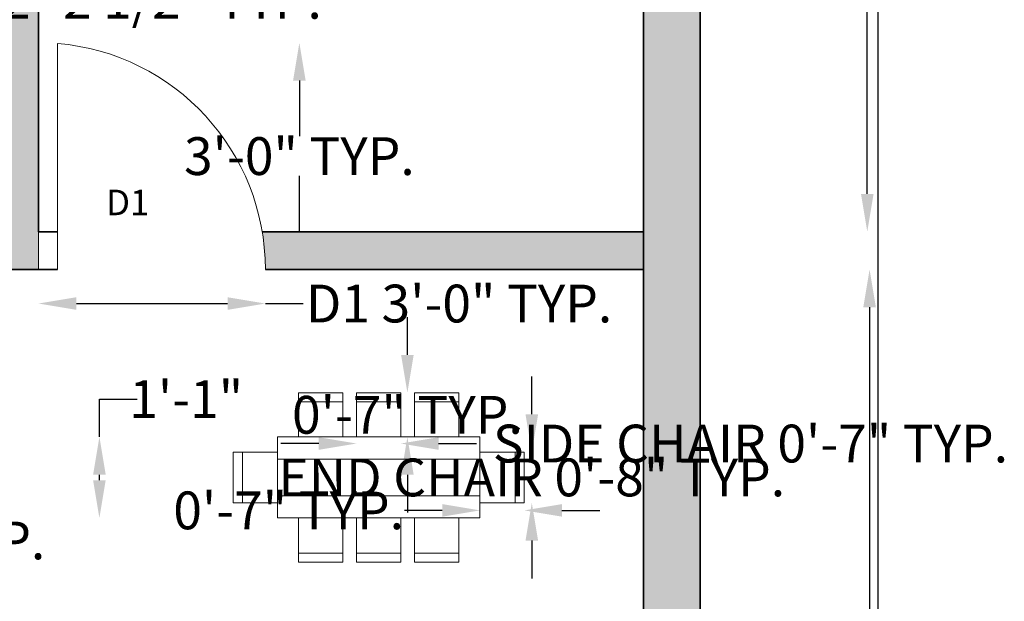
# Model space of a CAD drawing. Units: inches. Extents: x 2178 to 3409, y 1711 to 2279.
# Tile 4 of 8: x 2368 to 2524, y 2047 to 2140. Entities that reach past the tile are written whole.
import ezdxf

# ---------------------------------------------------------------- set-up
doc = ezdxf.new("R2010")
doc.units = ezdxf.units.IN
for name, color, linetype, lineweight in [('A-ANNO-DIMS', 2, 'Continuous', 18), ('A-ANNO-IDEN', 3, 'Continuous', 18), ('A-DOOR', 4, 'Continuous', 18), ('A-FURN', 8, 'Continuous', 18), ('A-WALL', 7, 'Continuous', 35), ('A-WALL-PATT', 252, 'Continuous', 13)]:
    doc.layers.add(name, color=color, linetype=linetype, lineweight=lineweight)
doc.styles.get("Standard").update_dxf_attribs({"font": 'arial.ttf'})
doc.dimstyles.get("Standard").update_dxf_attribs({"dimtxt": 6, "dimasz": 6, "dimexe": 0.18, "dimexo": 0.0625, "dimgap": 0.09, "dimtad": 0, "dimtih": 1, "dimtoh": 1, "dimdec": 4, "dimzin": 0, "dimdsep": 46, "dimlunit": 4, "dimtxsty": 'Standard', "dimcen": 0.09, "dimse1": 1, "dimse2": 1, "dimadec": 0, "dimazin": 0, "dimtfac": 1, "dimtdec": 4, "dimtofl": 0, "dimtmove": 0, "dimatfit": 3, "dimfxl": 1, "dimtolj": 1, "dimtzin": 0, "dimarcsym": 0})

# ---------------------------------------------------------------- blocks, each defined once
blk = doc.blocks.new('*D21')
at = {"layer": 'A-ANNO-DIMS', "color": 0, "lineweight": -2, "transparency": 16777216}
for p, q in [((2502.61, 2232.04), (2502.61, 2175.14)), ((2502.61, 2112.04), (2502.61, 2168.94))]:
    blk.add_line(p, q, dxfattribs=at)
at = {"layer": 'A-ANNO-DIMS', "color": 0, "transparency": 16777216}
for points in [[(2501.61, 2232.04), (2503.61, 2232.04), (2502.61, 2238.04)], [(2501.61, 2112.04), (2503.61, 2112.04), (2502.61, 2106.04)]]:
    blk.add_solid(points, dxfattribs=at)
at = {"layer": 'Defpoints', "color": 0, "transparency": 16777216}
for p in [(2467.06, 2238.04), (2467.06, 2106.04), (2502.61, 2106.04)]:
    blk.add_point(p, dxfattribs=at)
at = {"layer": 'A-ANNO-DIMS', "color": 0, "transparency": 16777216, "insert": (2502.61, 2172.04), "char_height": 6, "attachment_point": 5}
blk.add_mtext("\\A1;11'", dxfattribs=at)
blk = doc.blocks.new('*D22')
at = {"layer": 'A-ANNO-DIMS', "color": 0, "lineweight": -2, "transparency": 16777216}
for p, q in [((2502.98, 2094.04), (2502.98, 1959.14)), ((2502.98, 1818.04), (2502.98, 1952.94))]:
    blk.add_line(p, q, dxfattribs=at)
at = {"layer": 'A-ANNO-DIMS', "color": 0, "transparency": 16777216}
for points in [[(2501.98, 2094.04), (2503.98, 2094.04), (2502.98, 2100.04)], [(2501.98, 1818.04), (2503.98, 1818.04), (2502.98, 1812.04)]]:
    blk.add_solid(points, dxfattribs=at)
at = {"layer": 'Defpoints', "color": 0, "transparency": 16777216}
for p in [(2467.06, 2100.04), (2467.06, 1812.04), (2502.98, 1812.04)]:
    blk.add_point(p, dxfattribs=at)
at = {"layer": 'A-ANNO-DIMS', "color": 0, "transparency": 16777216, "insert": (2502.98, 1956.04), "char_height": 6, "attachment_point": 5}
blk.add_mtext("\\A1;24'", dxfattribs=at)
blk = doc.blocks.new('DINING-CHAIR-SIDE')
for p, q in [((0, 7.02), (0, 0)), ((7.02, 7.02), (0, 7.02)), ((7.02, 0), (7.02, 7.02)), ((0, 5.56), (7.02, 5.56))]:
    blk.add_line(p, q)
blk = doc.blocks.new('DINING-CHAIR-END')
for p, q in [((0, 0), (0, 8.04)), ((0, 8.04), (7.02, 8.04)), ((1.46, 8.04), (1.46, 0)), ((7.02, 0), (0, 0))]:
    blk.add_line(p, q)
blk = doc.blocks.new('DOOR-36')
for p, q in [((0, 0), (0, 36)), ((3, 0), (3, 35.87)), ((3, 0), (0, 0))]:
    blk.add_line(p, q)
blk.add_arc((0, 0), 36, 0, 85.2198)
blk = doc.blocks.new('*D38')
at = {"layer": 'A-ANNO-DIMS', "color": 0, "lineweight": -2, "transparency": 16777216}
for p, q in [((2338.85, 2142.85), (2353.23, 2142.85)), ((2359.23, 2142.85), (2365.23, 2142.85))]:
    blk.add_line(p, q, dxfattribs=at)
at = {"layer": 'A-ANNO-DIMS', "color": 0, "transparency": 16777216}
for points in [[(2338.85, 2143.85), (2338.85, 2141.85), (2332.85, 2142.85)], [(2353.23, 2143.85), (2353.23, 2141.85), (2359.23, 2142.85)]]:
    blk.add_solid(points, dxfattribs=at)
at = {"layer": 'Defpoints', "color": 0, "transparency": 16777216}
for p in [(2332.85, 2152.21), (2359.23, 2152.21), (2359.23, 2142.85)]:
    blk.add_point(p, dxfattribs=at)
at = {"layer": 'A-ANNO-DIMS', "color": 0, "transparency": 16777216, "insert": (2390.65, 2142.85), "char_height": 6, "attachment_point": 5}
blk.add_mtext('\\A1;2\'-2 1/2" TYP.', dxfattribs=at)
blk = doc.blocks.new('*D39')
at = {"layer": 'A-ANNO-DIMS', "color": 0, "lineweight": -2, "transparency": 16777216}
for p, q in [((2415.54, 2072.42), (2409.54, 2072.42)), ((2434.56, 2072.42), (2440.56, 2072.42))]:
    blk.add_line(p, q, dxfattribs=at)
at = {"layer": 'A-ANNO-DIMS', "color": 0, "transparency": 16777216}
for points in [[(2415.54, 2073.42), (2415.54, 2071.42), (2421.54, 2072.42)], [(2434.56, 2073.42), (2434.56, 2071.42), (2428.56, 2072.42)]]:
    blk.add_solid(points, dxfattribs=at)
at = {"layer": 'Defpoints', "color": 0, "transparency": 16777216}
for p in [(2421.54, 2073.47), (2428.56, 2073.47), (2428.56, 2072.42)]:
    blk.add_point(p, dxfattribs=at)
at = {"layer": 'A-ANNO-DIMS', "color": 0, "transparency": 16777216, "insert": (2484.07, 2072.42), "char_height": 6, "attachment_point": 5}
blk.add_mtext('\\A1;SIDE CHAIR 0\'-7" TYP.', dxfattribs=at)
blk = doc.blocks.new('*D40')
at = {"layer": 'A-ANNO-DIMS', "color": 0, "lineweight": -2, "transparency": 16777216}
for p, q in [((2429.61, 2086.49), (2429.61, 2092.49)), ((2429.61, 2067.47), (2429.61, 2061.47))]:
    blk.add_line(p, q, dxfattribs=at)
at = {"layer": 'A-ANNO-DIMS', "color": 0, "transparency": 16777216}
for points in [[(2428.61, 2086.49), (2430.61, 2086.49), (2429.61, 2080.49)], [(2428.61, 2067.47), (2430.61, 2067.47), (2429.61, 2073.47)]]:
    blk.add_solid(points, dxfattribs=at)
at = {"layer": 'Defpoints', "color": 0, "transparency": 16777216}
for p in [(2428.56, 2080.49), (2429.61, 2080.49), (2428.56, 2073.47)]:
    blk.add_point(p, dxfattribs=at)
at = {"layer": 'A-ANNO-DIMS', "color": 0, "transparency": 16777216, "insert": (2429.61, 2076.98), "char_height": 6, "attachment_point": 5}
blk.add_mtext('\\A1;0\'-7" TYP.', dxfattribs=at)
blk = doc.blocks.new('*D41')
at = {"layer": 'A-ANNO-DIMS', "color": 0, "lineweight": -2, "transparency": 16777216}
for p, q in [((2449.36, 2077.06), (2449.36, 2083.06)), ((2449.36, 2057.02), (2449.36, 2051.02))]:
    blk.add_line(p, q, dxfattribs=at)
at = {"layer": 'A-ANNO-DIMS', "color": 0, "transparency": 16777216}
for points in [[(2448.36, 2077.06), (2450.36, 2077.06), (2449.36, 2071.06)], [(2448.36, 2057.02), (2450.36, 2057.02), (2449.36, 2063.02)]]:
    blk.add_solid(points, dxfattribs=at)
at = {"layer": 'Defpoints', "color": 0, "transparency": 16777216}
for p in [(2448.15, 2071.06), (2448.15, 2063.02), (2449.36, 2063.02)]:
    blk.add_point(p, dxfattribs=at)
at = {"layer": 'A-ANNO-DIMS', "color": 0, "transparency": 16777216, "insert": (2449.36, 2067.04), "char_height": 6, "attachment_point": 5}
blk.add_mtext('\\A1;END CHAIR 0\'-8" TYP.', dxfattribs=at)
blk = doc.blocks.new('*D42')
at = {"layer": 'A-ANNO-DIMS', "color": 0, "lineweight": -2, "transparency": 16777216}
for p, q in [((2435.13, 2061.81), (2429.13, 2061.81)), ((2454.15, 2061.81), (2460.15, 2061.81))]:
    blk.add_line(p, q, dxfattribs=at)
at = {"layer": 'A-ANNO-DIMS', "color": 0, "transparency": 16777216}
for points in [[(2435.13, 2062.81), (2435.13, 2060.81), (2441.13, 2061.81)], [(2454.15, 2062.81), (2454.15, 2060.81), (2448.15, 2061.81)]]:
    blk.add_solid(points, dxfattribs=at)
at = {"layer": 'Defpoints', "color": 0, "transparency": 16777216}
for p in [(2441.13, 2063.02), (2441.13, 2061.81), (2448.15, 2063.02)]:
    blk.add_point(p, dxfattribs=at)
at = {"layer": 'A-ANNO-DIMS', "color": 0, "transparency": 16777216, "insert": (2410.76, 2061.81), "char_height": 6, "attachment_point": 5}
blk.add_mtext('\\A1;0\'-7" TYP.', dxfattribs=at)
blk = doc.blocks.new('*D53')
at = {"layer": 'A-ANNO-DIMS', "color": 0, "lineweight": -2, "transparency": 16777216}
for p, q in [((2293.06, 2057.04), (2311.06, 2057.04)), ((2317.06, 2057.04), (2323.06, 2057.04))]:
    blk.add_line(p, q, dxfattribs=at)
at = {"layer": 'A-ANNO-DIMS', "color": 0, "transparency": 16777216}
for points in [[(2293.06, 2058.04), (2293.06, 2056.04), (2287.06, 2057.04)], [(2311.06, 2058.04), (2311.06, 2056.04), (2317.06, 2057.04)]]:
    blk.add_solid(points, dxfattribs=at)
at = {"layer": 'Defpoints', "color": 0, "transparency": 16777216}
for p in [(2287.06, 2061.54), (2317.06, 2061.54), (2317.06, 2057.04)]:
    blk.add_point(p, dxfattribs=at)
at = {"layer": 'A-ANNO-DIMS', "color": 0, "transparency": 16777216, "insert": (2347.81, 2057.04), "char_height": 6, "attachment_point": 5}
blk.add_mtext('\\A1;D2 2\'-6" TYP.', dxfattribs=at)
blk = doc.blocks.new('*D55')
at = {"layer": 'A-ANNO-DIMS', "color": 0, "lineweight": -2, "transparency": 16777216}
for p, q in [((2377.06, 2094.64), (2401.06, 2094.64)), ((2407.06, 2094.64), (2413.06, 2094.64))]:
    blk.add_line(p, q, dxfattribs=at)
at = {"layer": 'A-ANNO-DIMS', "color": 0, "transparency": 16777216}
for points in [[(2377.06, 2095.64), (2377.06, 2093.64), (2371.06, 2094.64)], [(2401.06, 2095.64), (2401.06, 2093.64), (2407.06, 2094.64)]]:
    blk.add_solid(points, dxfattribs=at)
at = {"layer": 'Defpoints', "color": 0, "transparency": 16777216}
for p in [(2371.06, 2100.04), (2407.06, 2100.04), (2407.06, 2094.64)]:
    blk.add_point(p, dxfattribs=at)
at = {"layer": 'A-ANNO-DIMS', "color": 0, "transparency": 16777216, "insert": (2437.81, 2094.64), "char_height": 6, "attachment_point": 5}
blk.add_mtext('\\A1;D1 3\'-0" TYP.', dxfattribs=at)
blk = doc.blocks.new('*D56')
at = {"layer": 'A-ANNO-DIMS', "color": 0, "lineweight": -2, "transparency": 16777216}
for p, q in [((2412.46, 2130.04), (2412.46, 2121.2)), ((2412.46, 2106.04), (2412.46, 2114.89))]:
    blk.add_line(p, q, dxfattribs=at)
at = {"layer": 'A-ANNO-DIMS', "color": 0, "transparency": 16777216}
for points in [[(2411.46, 2130.04), (2413.46, 2130.04), (2412.46, 2136.04)], [(2411.46, 2106.04), (2413.46, 2106.04), (2412.46, 2100.04)]]:
    blk.add_solid(points, dxfattribs=at)
at = {"layer": 'Defpoints', "color": 0, "transparency": 16777216}
for p in [(2407.06, 2136.04), (2412.46, 2136.04), (2407.06, 2100.04)]:
    blk.add_point(p, dxfattribs=at)
at = {"layer": 'A-ANNO-DIMS', "color": 0, "transparency": 16777216, "insert": (2412.46, 2118.04), "char_height": 6, "attachment_point": 5}
blk.add_mtext('\\A1;3\'-0" TYP.', dxfattribs=at)
blk = doc.blocks.new('*D66')
at = {"layer": 'A-ANNO-DIMS', "color": 0, "lineweight": -2, "transparency": 16777216}
for p, q in [((2414.97, 2032.35), (2416.94, 2032.35)), ((2435.13, 2032.35), (2433.17, 2032.35))]:
    blk.add_line(p, q, dxfattribs=at)
at = {"layer": 'A-ANNO-DIMS', "color": 0, "transparency": 16777216}
for points in [[(2414.97, 2033.35), (2414.97, 2031.35), (2408.97, 2032.35)], [(2435.13, 2033.35), (2435.13, 2031.35), (2441.13, 2032.35)]]:
    blk.add_solid(points, dxfattribs=at)
at = {"layer": 'Defpoints', "color": 0, "transparency": 16777216}
for p in [(2408.97, 2060.6), (2441.13, 2060.6), (2408.97, 2032.35)]:
    blk.add_point(p, dxfattribs=at)
at = {"layer": 'A-ANNO-DIMS', "color": 0, "transparency": 16777216, "insert": (2425.05, 2032.35), "char_height": 6, "attachment_point": 5}
blk.add_mtext('\\A1;2\'-8"', dxfattribs=at)
blk = doc.blocks.new('*D67')
at = {"layer": 'A-ANNO-DIMS', "color": 0, "lineweight": -2, "transparency": 16777216}
for p, q in [((2380.72, 2073.47), (2380.72, 2079.47)), ((2380.72, 2079.47), (2386.72, 2079.47)), ((2380.72, 2066.6), (2380.72, 2067.47))]:
    blk.add_line(p, q, dxfattribs=at)
at = {"layer": 'A-ANNO-DIMS', "color": 0, "transparency": 16777216}
for points in [[(2379.72, 2067.47), (2381.72, 2067.47), (2380.72, 2073.47)], [(2379.72, 2066.6), (2381.72, 2066.6), (2380.72, 2060.6)]]:
    blk.add_solid(points, dxfattribs=at)
at = {"layer": 'Defpoints', "color": 0, "transparency": 16777216}
for p in [(2380.72, 2073.47), (2408.97, 2073.47), (2408.97, 2060.6)]:
    blk.add_point(p, dxfattribs=at)
at = {"layer": 'A-ANNO-DIMS', "color": 0, "transparency": 16777216, "insert": (2394.5, 2079.47), "char_height": 6, "attachment_point": 5}
blk.add_mtext('\\A1;1\'-1"', dxfattribs=at)
blk = doc.blocks.new('*D71')
at = {"layer": 'A-ANNO-DIMS', "color": 0, "lineweight": -2, "transparency": 16777216}
for p, q in [((2381.625685, 2275.292563), (2375.625685, 2275.292563)), ((2410.582731, 2275.292563), (2416.582731, 2275.292563))]:
    blk.add_line(p, q, dxfattribs=at)
at = {"layer": 'A-ANNO-DIMS', "color": 0, "transparency": 16777216}
for points in [[(2381.625685, 2276.292563), (2381.625685, 2274.292563), (2387.625685, 2275.292563)], [(2410.582731, 2276.292563), (2410.582731, 2274.292563), (2404.582731, 2275.292563)]]:
    blk.add_solid(points, dxfattribs=at)
at = {"layer": 'Defpoints', "color": 0, "transparency": 16777216}
for p in [(2404.582731, 2275.292563), (2387.625685, 1942.827852), (2404.582731, 1942.827852)]:
    blk.add_point(p, dxfattribs=at)
at = {"layer": 'A-ANNO-DIMS', "color": 0, "transparency": 16777216, "insert": (2396.104208, 2275.292563), "char_height": 6, "attachment_point": 5}
blk.add_mtext('\\A1;1\'-5"', dxfattribs=at)
blk = doc.blocks.new('*D73')
at = {"layer": 'A-ANNO-DIMS', "color": 0, "lineweight": -2, "transparency": 16777216}
for p, q in [((2387.37, 2275.29), (2388.32, 2275.29)), ((2405.5, 2275.29), (2404.55, 2275.29))]:
    blk.add_line(p, q, dxfattribs=at)
at = {"layer": 'A-ANNO-DIMS', "color": 0, "transparency": 16777216}
for points in [[(2387.37, 2276.29), (2387.37, 2274.29), (2381.37, 2275.29)], [(2405.5, 2276.29), (2405.5, 2274.29), (2411.5, 2275.29)]]:
    blk.add_solid(points, dxfattribs=at)
at = {"layer": 'Defpoints', "color": 0, "transparency": 16777216}
for p in [(2411.5, 2275.29), (2381.37, 1966.49), (2411.5, 1966.49)]:
    blk.add_point(p, dxfattribs=at)
at = {"layer": 'A-ANNO-DIMS', "color": 0, "transparency": 16777216, "insert": (2396.44, 2275.29), "char_height": 6, "attachment_point": 5}
blk.add_mtext('\\A1;2\'-6"', dxfattribs=at)
blk = doc.blocks.new('*D75')
at = {"layer": 'A-ANNO-DIMS', "color": 0, "lineweight": -2, "transparency": 16777216}
for p, q in [((2504.31, 2241.04), (2504.31, 1998.2)), ((2504.31, 1749.04), (2504.31, 1991.89))]:
    blk.add_line(p, q, dxfattribs=at)
at = {"layer": 'A-ANNO-DIMS', "color": 0, "transparency": 16777216}
for points in [[(2503.31, 2241.04), (2505.31, 2241.04), (2504.31, 2247.04)], [(2503.31, 1749.04), (2505.31, 1749.04), (2504.31, 1743.04)]]:
    blk.add_solid(points, dxfattribs=at)
at = {"layer": 'Defpoints', "color": 0, "transparency": 16777216}
for p in [(2476.06, 2247.04), (2504.31, 2247.04), (2476.06, 1743.04)]:
    blk.add_point(p, dxfattribs=at)
at = {"layer": 'A-ANNO-DIMS', "color": 0, "transparency": 16777216, "insert": (2504.31, 1995.04), "char_height": 6, "attachment_point": 5}
blk.add_mtext('\\A1;42\'-0"', dxfattribs=at)

msp = doc.modelspace()

# ---------------------------------------------------------------- hatches: boundary and pattern name
at = {"layer": 'A-WALL-PATT'}
h = msp.add_hatch(color=256, dxfattribs=at)
h.dxf.hatch_style = 1
h.paths.add_polyline_path([(2233.06485, 1992.04256), (2317.06485, 1992.04256), (2317.06485, 1998.04256), (2317.06485, 2006.75072), (2311.06485, 2006.75072), (2311.06485, 1998.04256), (2233.06485, 1998.04256), (2233.06485, 2009.64251), (2224.06485, 2009.64251), (2224.06485, 1863.04256), (2233.06485, 1863.04256), (2278.65041, 1863.04256), (2278.65041, 1872.04256), (2233.06485, 1872.04256)])
h.paths.add_polyline_path([(2359.06485, 1992.04256), (2359.06485, 1998.04256), (2353.06485, 1998.04256), (2353.06485, 1962.04256), (2353.06485, 1872.04256), (2314.65041, 1872.04256), (2314.65041, 1863.04256), (2359.06485, 1863.04256), (2359.06485, 1872.04256)])
h.paths.add_polyline_path([(2401.06485, 1890.04256), (2371.06485, 1890.04256), (2359.06485, 1890.04256), (2359.06485, 1884.04256), (2371.06485, 1884.04256), (2377.06485, 1884.04256), (2401.06485, 1884.04256)])
h.paths.add_polyline_path([(2353.06485, 1802.77269), (2359.06485, 1802.77269), (2359.06485, 1808.77269), (2356.83755, 1808.77269), (2353.06485, 1808.77269), (2347.91295, 1808.77269), (2347.91295, 1802.77269), (2347.91295, 1749.04256), (2342.02347, 1749.04256), (2342.02347, 1743.04256), (2353.06485, 1743.04256)])
h.paths.add_polyline_path([(2476.06485, 2247.04256), (2442.91353, 2247.04256), (2442.91353, 2238.04256), (2467.06485, 2238.04256), (2467.06485, 2041.93675), (2476.06485, 2041.93675)])
h.paths.add_polyline_path([(2467.06485, 2106.04256), (2406.56133, 2106.04256, -0.04188649), (2407.06485, 2100.04256), (2467.06485, 2100.04256)])
h.paths.add_polyline_path([(2406.91353, 2247.04256), (2321.22384, 2247.04256), (2321.22384, 2238.04256), (2365.06485, 2238.04256), (2365.06485, 2106.04256), (2365.06485, 2100.04256), (2371.06485, 2100.04256), (2371.06485, 2136.04256), (2371.06485, 2238.04256), (2406.91353, 2238.04256)])
h.paths.add_polyline_path([(2285.22384, 2247.04256), (2224.06485, 2247.04256), (2224.06485, 2087.1459), (2233.06485, 2087.1459), (2233.06485, 2100.04256), (2329.06485, 2100.04256, -0.04188649), (2329.56837, 2106.04256), (2233.06485, 2106.04256), (2233.06485, 2238.04256), (2285.22384, 2238.04256)])
h.paths.add_polyline_path([(2317.06485, 2052.04256), (2317.06485, 2061.5418), (2311.06485, 2061.5418), (2311.06485, 2052.04256), (2233.06485, 2052.04256), (2233.06485, 2063.1459), (2224.06485, 2063.1459), (2224.06485, 2033.64251), (2233.06485, 2033.64251), (2233.06485, 2046.04256), (2311.06485, 2046.04256), (2311.06485, 2036.1446, -0.050382044), (2317.06485, 2036.75072), (2317.06485, 2046.04256)])

# ---------------------------------------------------------------- linework, layer by layer
at = {"layer": 'A-FURN'}
for p, q in [((2408.97204, 2073.46856), (2441.13383, 2073.46856)), ((2408.97204, 2060.60384), (2408.97204, 2073.46856)), ((2441.13383, 2073.46856), (2441.13383, 2060.60384)), ((2408.97204, 2069.96), (2441.13383, 2069.96)), ((2408.97204, 2064.1124), (2441.13383, 2064.1124)), ((2441.13383, 2060.60384), (2408.97204, 2060.60384))]:
    msp.add_line(p, q, dxfattribs=at)
at = {"layer": 'A-WALL'}
for p, q in [((2476.06485, 2247.04256), (2476.06485, 1803.04256)), ((2371.06485, 2238.04256), (2371.06485, 2106.04256)), ((2467.06485, 2238.04256), (2467.06485, 1812.04256)), ((2371.06485, 2106.04256), (2374.06485, 2106.04256)), ((2406.56133, 2106.04256), (2467.06485, 2106.04256)), ((2365.06485, 2100.04256), (2371.06485, 2100.04256)), ((2371.06485, 2100.04256), (2374.06485, 2100.04256)), ((2407.06485, 2100.04256), (2467.06485, 2100.04256))]:
    msp.add_line(p, q, dxfattribs=at)

# ---------------------------------------------------------------- block references
at = {"layer": 'A-DOOR'}
msp.add_blockref('DOOR-36', (2371.06485, 2100.04256), dxfattribs=at)
at = {"layer": 'A-FURN'}
for name, p in [('DINING-CHAIR-SIDE', (2412.33441, 2073.46856)), ('DINING-CHAIR-SIDE', (2421.54438, 2073.46856)), ('DINING-CHAIR-SIDE', (2430.75434, 2073.46856)), ('DINING-CHAIR-END', (2401.95492, 2063.01597))]:
    msp.add_blockref(name, p, dxfattribs=at)
at = {"layer": 'A-FURN', "rotation": 180}
for name, p in [('DINING-CHAIR-END', (2448.15095, 2071.05642)), ('DINING-CHAIR-SIDE', (2419.35153, 2060.60384)), ('DINING-CHAIR-SIDE', (2428.56149, 2060.60384)), ('DINING-CHAIR-SIDE', (2437.77146, 2060.60384))]:
    msp.add_blockref(name, p, dxfattribs=at)

# ---------------------------------------------------------------- texts
at = {"layer": 'A-ANNO-IDEN', "insert": (2381.78025, 2112.7087), "char_height": 4.051205, "attachment_point": 1}
msp.add_mtext_dynamic_manual_height_columns('D1', width=167.0263497, gutter_width=20.25603, heights=[0], dxfattribs=at)

# ---------------------------------------------------------------- dimensions: what is measured, and where the dimension line sits
at = {"layer": 'A-ANNO-DIMS'}
for base, p1, p2, picture, middle in [((2404.58273, 2275.29256), (2387.62568, 1942.82785), (2404.58273, 1942.82785), '*D71', (2396.10421, 2275.29256)), ((2411.50157, 2275.29256), (2381.37394, 1966.48789), (2411.50157, 1966.48789), '*D73', (2396.43775, 2275.29256))]:
    dim = msp.add_linear_dim(base=base, p1=p1, p2=p2, dimstyle='Standard', override={"dimdec": 1, "dimlfac": 1, "dimrnd": 0, "dimzin": 1, "dimdsep": 46, "dimlunit": 4, "dimfrac": 2}, dxfattribs=at)
    dim.commit()
    dim.dimension.update_dxf_attribs({"geometry": picture, "text_midpoint": middle})
for base, p1, p2, angle, override, picture, middle in [((2504.31485, 2247.04256), (2476.06485, 1743.04256), (2476.06485, 2247.04256), 90, {"dimdec": 1, "dimlfac": 1, "dimrnd": 0, "dimzin": 1, "dimdsep": 46, "dimlunit": 4, "dimfrac": 2}, '*D75', (2504.31485, 1995.04256)), ((2502.61341, 2106.04256), (2467.06485, 2238.04256), (2467.06485, 2106.04256), 90, {"dimclrd": 0, "dimclre": 0, "dimclrt": 0}, '*D21', (2502.61341, 2172.04256)), ((2502.97839, 1812.04256), (2467.06485, 2100.04256), (2467.06485, 1812.04256), 90, {"dimclrd": 0, "dimclre": 0, "dimclrt": 0}, '*D22', (2502.97839, 1956.04256)), ((2380.72204, 2073.46856), (2408.97204, 2060.60384), (2408.97204, 2073.46856), 90, {"dimdec": 1, "dimlfac": 1, "dimrnd": 0, "dimzin": 1, "dimdsep": 46, "dimlunit": 4, "dimfrac": 2}, '*D67', (2394.5044, 2079.46856)), ((2408.97204, 2032.35384), (2441.13383, 2060.60384), (2408.97204, 2060.60384), 180, {"dimdec": 1, "dimlfac": 1, "dimrnd": 0, "dimzin": 1, "dimdsep": 46, "dimlunit": 4, "dimfrac": 2}, '*D66', (2425.05294, 2032.35384))]:
    dim = msp.add_linear_dim(base=base, p1=p1, p2=p2, angle=angle, dimstyle='Standard', override=override, dxfattribs=at)
    dim.commit()
    dim.dimension.update_dxf_attribs({"geometry": picture, "text_midpoint": middle})
for base, p1, p2, text, picture, middle in [((2359.23207, 2142.84918), (2332.85429, 2152.20941), (2359.23207, 2152.20941), '<> TYP.', '*D38', (2390.65017, 2142.84918)), ((2407.06485, 2094.64256), (2371.06485, 2100.04256), (2407.06485, 2100.04256), 'D1 <> TYP.', '*D55', (2437.81378, 2094.64256)), ((2428.56149, 2072.41599), (2421.54438, 2073.46856), (2428.56149, 2073.46856), 'SIDE CHAIR <> TYP.', '*D39', (2484.07373, 2072.41599)), ((2317.06485, 2057.0418), (2287.06485, 2061.5418), (2317.06485, 2061.5418), 'D2 <> TYP.', '*D53', (2347.81378, 2057.0418))]:
    dim = msp.add_linear_dim(base=base, p1=p1, p2=p2, text=text, dimstyle='Standard', override={"dimdec": 1, "dimlfac": 1, "dimrnd": 0, "dimzin": 1, "dimdsep": 46, "dimlunit": 4, "dimfrac": 2}, dxfattribs=at)
    dim.commit()
    dim.dimension.update_dxf_attribs({"geometry": picture, "text_midpoint": middle})
for base, p1, p2, angle, text, picture, middle in [((2412.46485, 2136.04256), (2407.06485, 2100.04256), (2407.06485, 2136.04256), 90, '<> TYP.', '*D56', (2412.46485, 2118.04256)), ((2429.61406, 2080.48568), (2428.56149, 2073.46856), (2428.56149, 2080.48568), 90, '<> TYP.', '*D40', (2429.61406, 2076.97712)), ((2449.35702, 2063.01597), (2448.15095, 2071.05642), (2448.15095, 2063.01597), 270, 'END CHAIR <> TYP.', '*D41', (2449.35702, 2067.0362)), ((2441.13383, 2061.80991), (2448.15095, 2063.01597), (2441.13383, 2063.01597), 180, '<> TYP.', '*D42', (2410.75734, 2061.80991))]:
    dim = msp.add_linear_dim(base=base, p1=p1, p2=p2, angle=angle, text=text, dimstyle='Standard', override={"dimdec": 1, "dimlfac": 1, "dimrnd": 0, "dimzin": 1, "dimdsep": 46, "dimlunit": 4, "dimfrac": 2}, dxfattribs=at)
    dim.commit()
    dim.dimension.update_dxf_attribs({"geometry": picture, "text_midpoint": middle})

doc.saveas('drawing.dxf')
